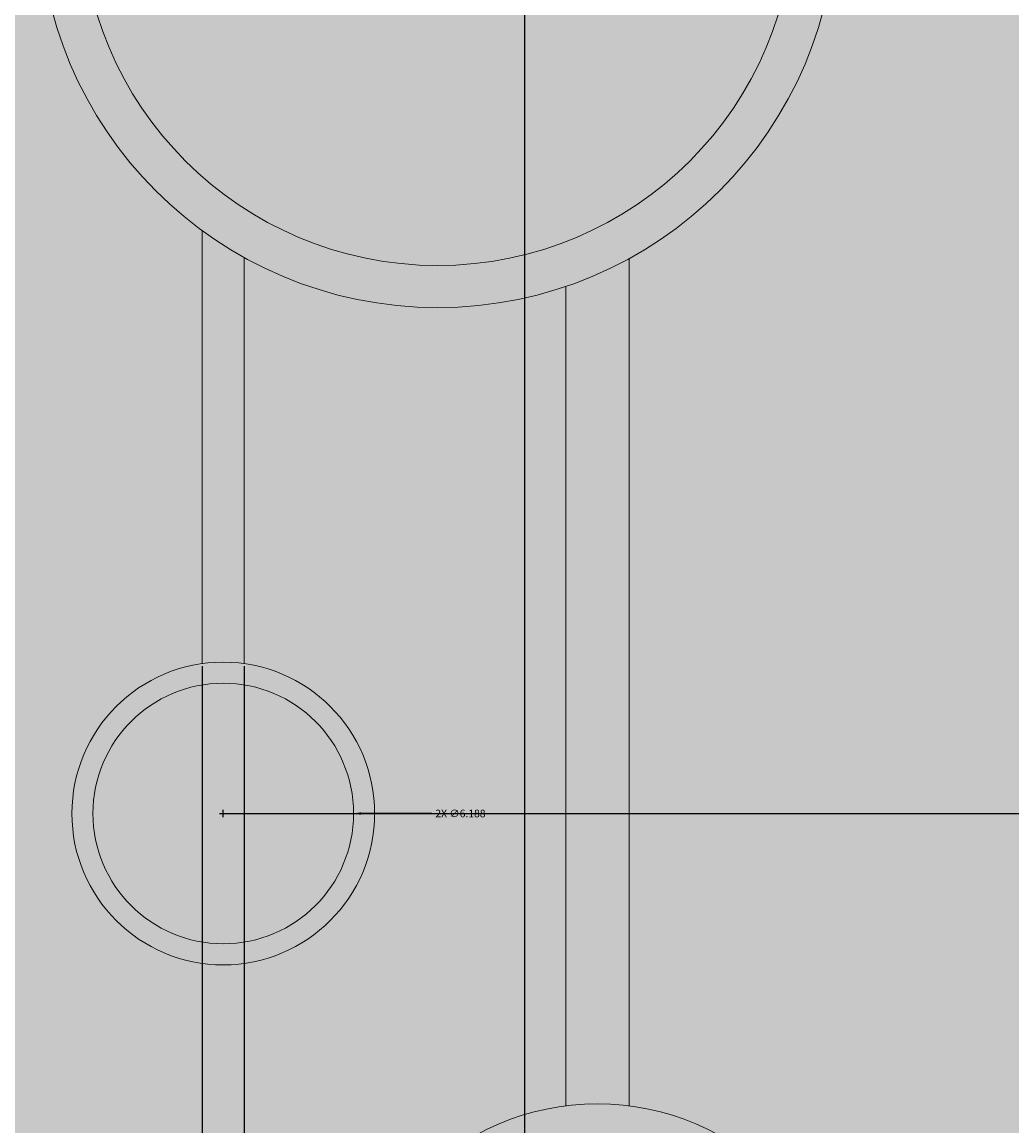
# Model space of a CAD drawing. Units: inches. Extents: x 4508 to 4723, y 847 to 1020.
# Tile 22 of 32: x 4657 to 4681, y 907 to 933. Entities that reach past the tile are written whole.
import ezdxf

# ---------------------------------------------------------------- set-up
doc = ezdxf.new("R2010")
doc.units = ezdxf.units.IN
for name, color, linetype, lineweight in [('A-ANNO-DIMS', 2, 'Continuous', 18), ('A-WALL-DECO', 6, 'Continuous', 18), ('A-WALL-PATT', 254, 'Continuous', 13)]:
    doc.layers.add(name, color=color, linetype=linetype, lineweight=lineweight)
doc.styles.get("Standard").update_dxf_attribs({"font": 'arial.ttf'})
doc.dimstyles.get("Standard").update_dxf_attribs({"dimtxt": 0.18, "dimasz": 0.18, "dimexe": 0.18, "dimexo": 0.0625, "dimgap": 0.09, "dimtad": 0, "dimtih": 1, "dimtoh": 1, "dimdec": 4, "dimzin": 0, "dimdsep": 46, "dimtxsty": 'Standard', "dimcen": 0.09, "dimadec": 0, "dimazin": 0, "dimtfac": 1, "dimtdec": 4, "dimtofl": 0, "dimtmove": 0, "dimatfit": 3, "dimfxl": 1, "dimtolj": 1, "dimtzin": 0, "dimarcsym": 0})

# ---------------------------------------------------------------- blocks, each defined once
blk = doc.blocks.new('*D13')
at = {"layer": 'A-ANNO-DIMS', "color": 0, "lineweight": -2, "transparency": 16777216}
for p, q in [((4669.325, 973.916), (4669.325, 866.617)), ((4689.994, 874.684), (4689.994, 866.617)), ((4669.505, 866.797), (4679.264, 866.797)), ((4689.814, 866.797), (4680.054, 866.797))]:
    blk.add_line(p, q, dxfattribs=at)
at = {"layer": 'A-ANNO-DIMS', "color": 0, "lineweight": 9, "transparency": 16777216}
for points in [[(4669.505, 866.827), (4669.505, 866.767), (4669.325, 866.797)], [(4689.814, 866.827), (4689.814, 866.767), (4689.994, 866.797)]]:
    blk.add_solid(points, dxfattribs=at)
at = {"layer": 'Defpoints', "color": 0, "lineweight": 9, "transparency": 16777216}
for p in [(4669.325, 973.978), (4689.994, 874.747), (4689.994, 866.797)]:
    blk.add_point(p, dxfattribs=at)
at = {"layer": 'A-ANNO-DIMS', "color": 0, "transparency": 16777216, "insert": (4679.659, 866.797), "char_height": 0.18, "attachment_point": 5}
blk.add_mtext('\\A1;20.67', dxfattribs=at)
blk = doc.blocks.new('*D15')
at = {"layer": 'A-ANNO-DIMS', "color": 0, "lineweight": -2, "transparency": 16777216}
for p, q in [((4661.671, 918.138), (4661.671, 866.617)), ((4662.671, 918.138), (4662.671, 866.617)), ((4661.851, 866.797), (4662.047, 866.797)), ((4662.491, 866.797), (4662.294, 866.797))]:
    blk.add_line(p, q, dxfattribs=at)
at = {"layer": 'A-ANNO-DIMS', "color": 0, "lineweight": 9, "transparency": 16777216}
for points in [[(4661.851, 866.827), (4661.851, 866.767), (4661.671, 866.797)], [(4662.491, 866.827), (4662.491, 866.767), (4662.671, 866.797)]]:
    blk.add_solid(points, dxfattribs=at)
at = {"layer": 'Defpoints', "color": 0, "lineweight": 9, "transparency": 16777216}
for p in [(4661.671, 918.2), (4662.671, 918.2), (4662.671, 866.797)]:
    blk.add_point(p, dxfattribs=at)
at = {"layer": 'A-ANNO-DIMS', "color": 0, "transparency": 16777216, "insert": (4662.171, 866.797), "char_height": 0.18, "attachment_point": 5}
blk.add_mtext('\\A1;1', dxfattribs=at)
blk = doc.blocks.new('*D19')
at = {"layer": 'A-ANNO-DIMS', "color": 0, "lineweight": -2, "transparency": 16777216}
for p, q in [((4662.233, 914.641), (4702.124, 914.641)), ((4701.944, 914.461), (4701.944, 908.376)), ((4701.944, 901.927), (4701.944, 908.012)), ((4671.119, 901.747), (4702.124, 901.747))]:
    blk.add_line(p, q, dxfattribs=at)
at = {"layer": 'A-ANNO-DIMS', "color": 0, "lineweight": 9, "transparency": 16777216}
for points in [[(4701.914, 914.461), (4701.974, 914.461), (4701.944, 914.641)], [(4701.914, 901.927), (4701.974, 901.927), (4701.944, 901.747)]]:
    blk.add_solid(points, dxfattribs=at)
at = {"layer": 'Defpoints', "color": 0, "lineweight": 9, "transparency": 16777216}
for p in [(4662.171, 914.641), (4701.944, 914.641), (4671.056, 901.747)]:
    blk.add_point(p, dxfattribs=at)
at = {"layer": 'A-ANNO-DIMS', "color": 0, "transparency": 16777216, "insert": (4701.944, 908.194), "char_height": 0.18, "attachment_point": 5}
blk.add_mtext('\\A1;12.894', dxfattribs=at)
blk = doc.blocks.new('*D20')
at = {"layer": 'A-ANNO-DIMS', "color": 0, "lineweight": -2, "transparency": 16777216}
for p, q in [((4667.324, 936.122), (4702.124, 936.122)), ((4701.944, 935.942), (4701.944, 925.563)), ((4701.944, 914.821), (4701.944, 925.2)), ((4662.233, 914.641), (4702.124, 914.641))]:
    blk.add_line(p, q, dxfattribs=at)
at = {"layer": 'A-ANNO-DIMS', "color": 0, "lineweight": 9, "transparency": 16777216}
for points in [[(4701.914, 935.942), (4701.974, 935.942), (4701.944, 936.122)], [(4701.914, 914.821), (4701.974, 914.821), (4701.944, 914.641)]]:
    blk.add_solid(points, dxfattribs=at)
at = {"layer": 'Defpoints', "color": 0, "lineweight": 9, "transparency": 16777216}
for p in [(4667.262, 936.122), (4701.944, 936.122), (4662.171, 914.641)]:
    blk.add_point(p, dxfattribs=at)
at = {"layer": 'A-ANNO-DIMS', "color": 0, "transparency": 16777216, "insert": (4701.944, 925.381), "char_height": 0.18, "attachment_point": 5}
blk.add_mtext('\\A1;21.48', dxfattribs=at)
blk = doc.blocks.new('*D47')
at = {"layer": 'A-ANNO-DIMS', "color": 0, "lineweight": -2, "transparency": 16777216}
for p, q in [((4662.171, 914.551), (4662.171, 914.731)), ((4662.081, 914.641), (4662.261, 914.641)), ((4667.121, 914.641), (4665.445, 914.641))]:
    blk.add_line(p, q, dxfattribs=at)
at = {"layer": 'A-ANNO-DIMS', "color": 0, "lineweight": 9, "transparency": 16777216}
blk.add_solid([(4665.445, 914.671), (4665.445, 914.611), (4665.265, 914.641)], dxfattribs=at)
at = {"layer": 'Defpoints', "color": 0, "lineweight": 9, "transparency": 16777216}
for p in [(4659.076, 914.641), (4665.265, 914.641)]:
    blk.add_point(p, dxfattribs=at)
at = {"layer": 'A-ANNO-DIMS', "color": 0, "transparency": 16777216, "insert": (4667.803, 914.641), "char_height": 0.18, "attachment_point": 5}
blk.add_mtext('\\A1;2X ∅6.188', dxfattribs=at)

msp = doc.modelspace()

# ---------------------------------------------------------------- hatches: boundary and pattern name
at = {"layer": 'A-WALL-PATT', "transparency": 33554508}
h = msp.add_hatch(color=256, dxfattribs=at)
h.dxf.hatch_style = 1
h.paths.add_polyline_path([(4661.6706, 954.043, -0.3739004), (4658.5765, 957.6021, -1), (4665.7646, 957.6021, -0.3739004), (4662.6706, 954.043), (4662.6706, 944.4021, -0.2114781), (4670.3062, 945.0869), (4670.3062, 968.0592, -0.4632086), (4663.3246, 973.9783, -0.4632086), (4670.3062, 979.8975), (4670.3062, 994.7469), (4588.9938, 994.7469), (4588.9938, 904.7469), (4657.9938, 904.7469), (4657.9938, 886.7469), (4549.9938, 886.7469), (4549.9938, 878.7469), (4693.9938, 878.7469), (4693.9938, 994.7469), (4671.8062, 994.7469), (4671.8062, 979.4411, -0.2941682), (4675.3246, 973.9783, -0.2941682), (4671.8062, 968.5156), (4671.8062, 944.4278, -0.2741114), (4676.7298, 936.1217, -0.2741114), (4671.8062, 927.8155), (4671.8062, 907.6998, -0.3779645), (4677.0562, 901.7469, -0.3779645), (4671.8062, 895.7939), (4671.8062, 883.7469), (4670.3062, 883.7469), (4670.3062, 895.7939, -0.3779645), (4665.0562, 901.7469, -0.3779645), (4670.3062, 907.6998), (4670.3062, 927.1564, -0.2114781), (4662.6706, 927.8412), (4662.6706, 918.2003, -0.3739004), (4665.7646, 914.6412, -1), (4658.5765, 914.6412, -0.3739004), (4661.6706, 918.2003), (4661.6706, 928.4807, -0.2391825), (4657.7936, 936.1217, -0.2391825), (4661.6706, 943.7626)])
at = {"layer": 'A-WALL-PATT', "transparency": 33554556}
h = msp.add_hatch(color=256, dxfattribs=at)
h.dxf.hatch_style = 1
h.paths.add_polyline_path([(4676.0562, 901.7469, 1), (4666.0562, 901.7469, 1)])
h.paths.add_polyline_path([(4659.0765, 914.6412, 1), (4665.2646, 914.6412, 1)])
h.paths.add_polyline_path([(4675.7298, 936.1217, 1), (4658.7936, 936.1217, 1)])
h.paths.add_polyline_path([(4659.0765, 957.6021, 1), (4665.2646, 957.6021, 1)])
h.paths.add_polyline_path([(4664.3246, 973.9783, 1), (4674.3246, 973.9783, 1)])
at = {"layer": 'A-WALL-PATT', "transparency": 33554681}
h = msp.add_hatch(color=256, dxfattribs=at)
h.dxf.hatch_style = 1
h.paths.add_polyline_path([(4676.7298, 936.1217, 1), (4657.7936, 936.1217, 1)])
h.paths.add_polyline_path([(4658.7936, 936.1217, -1), (4675.7298, 936.1217, -1)], flags=16)
h = msp.add_hatch(color=256, dxfattribs=at)
h.dxf.hatch_style = 1
h.paths.add_polyline_path([(4662.6706, 927.8412, -0.0313734), (4661.6706, 928.4807), (4661.6706, 918.2003, -0.0698991), (4662.6706, 918.2003)])
h = msp.add_hatch(color=256, dxfattribs=at)
h.dxf.hatch_style = 1
h.paths.add_polyline_path([(4671.8062, 927.8155, -0.0433429), (4670.3062, 927.1564), (4670.3062, 907.6998, -0.0627461), (4671.8062, 907.6998)])
h = msp.add_hatch(color=256, dxfattribs=at)
h.dxf.hatch_style = 1
h.paths.add_polyline_path([(4665.7646, 914.6412, 1), (4658.5765, 914.6412, 1)])
h.paths.add_polyline_path([(4659.0765, 914.6412, -1), (4665.2646, 914.6412, -1)], flags=16)
h = msp.add_hatch(color=256, dxfattribs=at)
h.dxf.hatch_style = 1
h.paths.add_polyline_path([(4677.0562, 901.7469, 1), (4665.0562, 901.7469, 1)])
h.paths.add_polyline_path([(4666.0562, 901.7469, -1), (4676.0562, 901.7469, -1)], flags=16)

# ---------------------------------------------------------------- linework, layer by layer
at = {"layer": 'A-WALL-DECO'}
for p, q in [((4671.8062, 907.6998), (4671.8062, 927.8155)), ((4670.3062, 927.1564), (4670.3062, 907.6998))]:
    msp.add_line(p, q, dxfattribs=at)
for points in [[(4661.6706, 928.4807), (4661.6706, 918.2003)], [(4662.6706, 918.2003), (4662.6706, 927.8412)]]:
    msp.add_lwpolyline(points, dxfattribs=at)
for centre, radius in [((4667.2617, 936.1217), 9.4681), ((4667.2617, 936.1217), 8.4681), ((4662.1706, 914.6412), 3.5941), ((4662.1706, 914.6412), 3.0941), ((4671.0562, 901.7469), 6)]:
    msp.add_circle(centre, radius, dxfattribs=at)

# ---------------------------------------------------------------- dimensions: what is measured, and where the dimension line sits
at = {"layer": 'A-ANNO-DIMS'}
for base, p1, p2, override, picture, middle in [((4689.9938, 866.7969), (4669.3246, 973.9783), (4689.9938, 874.7469), {"dimdec": 2, "dimlfac": 1, "dimrnd": 0, "dimzin": 0, "dimdsep": 46, "dimlunit": 2}, '*D13', (4679.6592, 866.7969)), ((4662.6706, 866.7969), (4661.6706, 918.2003), (4662.6706, 918.2003), {"dimdec": 0, "dimlfac": 1, "dimrnd": 0, "dimzin": 0, "dimdsep": 46, "dimlunit": 2}, '*D15', (4662.1706, 866.7969))]:
    dim = msp.add_linear_dim(base=base, p1=p1, p2=p2, dimstyle='Standard', override=override, dxfattribs=at)
    dim.commit()
    dim.dimension.update_dxf_attribs({"geometry": picture, "text_midpoint": middle})
for base, p1, p2, override, picture, middle in [((4701.9438, 936.1217), (4662.1706, 914.6412), (4667.2617, 936.1217), {"dimdec": 2, "dimlfac": 1, "dimrnd": 0, "dimzin": 0, "dimdsep": 46, "dimlunit": 2}, '*D20', (4701.9438, 925.3814)), ((4701.9438, 914.6412), (4671.0562, 901.7469), (4662.1706, 914.6412), {"dimdec": 3, "dimlfac": 1, "dimrnd": 0, "dimzin": 0, "dimdsep": 46, "dimlunit": 2}, '*D19', (4701.9438, 908.1941))]:
    dim = msp.add_linear_dim(base=base, p1=p1, p2=p2, angle=90, dimstyle='Standard', override=override, dxfattribs=at)
    dim.commit()
    dim.dimension.update_dxf_attribs({"geometry": picture, "text_midpoint": middle})
dim = msp.add_diameter_dim_2p(p1=(4659.0765, 914.6415), p2=(4665.2646, 914.641), text='2X <>', dimstyle='Standard', override={"dimdec": 3, "dimlfac": 1, "dimrnd": 0, "dimzin": 0, "dimdsep": 46, "dimlunit": 2}, dxfattribs=at)
dim.commit()
dim.dimension.update_dxf_attribs({"geometry": '*D47', "text_midpoint": (4667.1211, 914.6409), "dimtype": 163})

doc.saveas('drawing.dxf')
